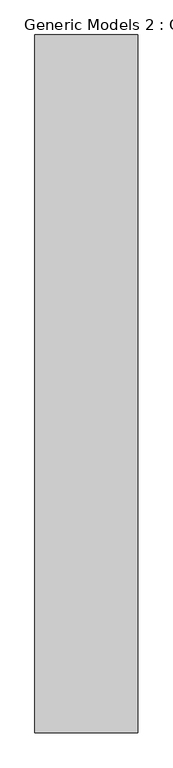
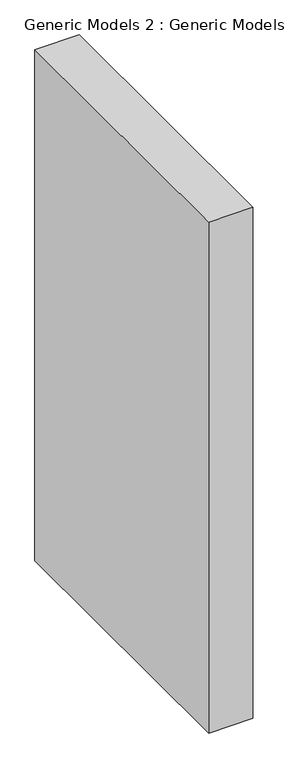
"""IFC4 building model written with IfcOpenShell, lengths in millimetres: proxy geometry, Generic Models 2 : Generic Models 2."""

from ifc_helpers import new_model, si_unit, origin, origin_with_axes, place, context, project, spatial, polyline, outline, extrude, source, transform, mapped, element, save


def generic_models_2_generic_models_2_14940448(model_context):
    return source(origin(), model_context, "Body", "SweptSolid", [
        extrude(outline(polyline([(-21617.0161422, -16342.7229916), (-21845.6161422, -16342.7229916), (-21845.6161422, -14789.9171312), (-21617.0161422, -14789.9171312), (-21617.0161422, -16342.7229916)])), origin_with_axes(), (0.0, 0.0, 1.0), 2789.0025902),
    ])


if __name__ == "__main__":
    model = new_model("IFC4")
    model_context = context("Model", 3, world=origin())
    ifc_project = project(units=[si_unit("LENGTHUNIT", "METRE", prefix="MILLI")], contexts=[model_context])
    site = spatial("IfcSite", under=ifc_project)
    building = spatial("IfcBuilding", under=site)
    placement = place(None, origin())
    generic_models_2_generic_models_2_shape = generic_models_2_generic_models_2_14940448(model_context)
    element("IfcBuildingElementProxy", 1, Name="Generic Models 2 : Generic Models 2", ObjectType="Generic Models 2 : Generic Models 2", at=placement, inside=building, context=model_context, shape_type="MappedRepresentation", body=[
        mapped(generic_models_2_generic_models_2_shape, transform((0.0, 0.0, 0.0), x_axis=(1.0, 0.0, 0.0), y_axis=(0.0, 1.0, 0.0), z_axis=(0.0, 0.0, 1.0))),
    ])
    save(model, "model.ifc")
